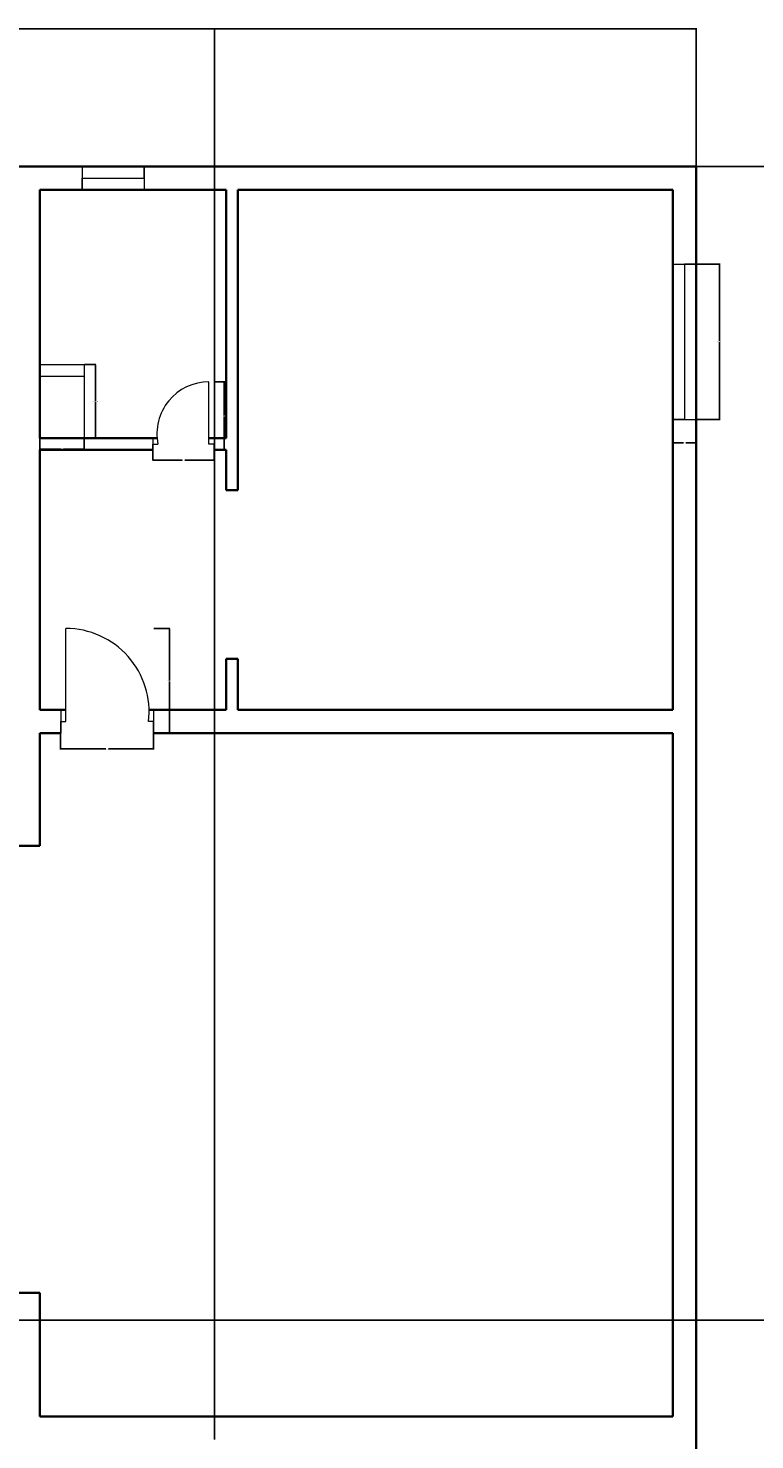
# Model space of a CAD drawing. Units: inches. Extents: x 2185 to 4426, y 1138 to 3073.
# Tile 12 of 14: x 3674 to 3955, y 1834 to 2380. Entities that reach past the tile are written whole.
import ezdxf

# ---------------------------------------------------------------- set-up
doc = ezdxf.new("R2010")
doc.units = ezdxf.units.IN
for name, color, linetype, lineweight in [('A-ANNO-DIMS', 2, 'Continuous', 18), ('A-ANNO-SYMB', 2, 'Continuous', 25), ('A-DOOR', 3, 'Continuous', 18), ('A-FLOR-CASE', 32, 'Continuous', 18), ('A-FURN', 8, 'Continuous', 18), ('A-GLAZ', 4, 'Continuous', 18), ('A-WALL', 7, 'Continuous', 35)]:
    doc.layers.add(name, color=color, linetype=linetype, lineweight=lineweight)
doc.styles.get("Standard").update_dxf_attribs({"font": 'arial.ttf'})
doc.dimstyles.get("Standard").update_dxf_attribs({"dimtxt": 0.18, "dimasz": 0.18, "dimexe": 0.18, "dimexo": 0.0625, "dimgap": 0.09, "dimtad": 0, "dimtih": 1, "dimtoh": 1, "dimdec": 4, "dimzin": 0, "dimdsep": 46, "dimtxsty": 'Standard', "dimcen": 0.09, "dimadec": 0, "dimazin": 0, "dimtfac": 1, "dimtdec": 4, "dimtofl": 0, "dimtmove": 0, "dimatfit": 3, "dimfxl": 1, "dimtolj": 1, "dimtzin": 0, "dimarcsym": 0})

# ---------------------------------------------------------------- blocks, each defined once
blk = doc.blocks.new('DOOR-SGL-24-ENSUITE')
for p, q in [((21.69, 2.25), (21.69, 26.25)), ((0, 4.5), (0, 0)), ((0, 0), (0, 2.25)), ((0, 2.25), (2, 2.25)), ((23.69, 2.25), (21.69, 2.25)), ((23.69, 4.5), (23.69, 0)), ((23.69, 0), (23.69, 2.25))]:
    blk.add_line(p, q)
blk.add_arc((21.69, 6.17), 20.08, 90, 191.26)
blk = doc.blocks.new('DOOR-SGL-36-BED-E')
for p, q in [((2, 4.5), (2, 40.5)), ((0, 9), (0, 0)), ((35.91, 9), (35.91, 0)), ((0, 0), (0, 4.5)), ((0, 4.5), (2, 4.5)), ((35.91, 4.5), (33.91, 4.5)), ((35.91, 0), (35.91, 4.5))]:
    blk.add_line(p, q)
blk.add_arc((2, 8.36), 32.14, 353.0978, 90)
blk = doc.blocks.new('WIN-PLAN-24IN-01')
for p, q in [((0, 9), (0, 0)), ((24, 4.5), (24, 9)), ((24, 9), (24, 0)), ((0, 0), (0, 4.5)), ((0, 4.5), (0, 4.5)), ((0, 4.5), (24, 4.5))]:
    blk.add_line(p, q)
blk = doc.blocks.new('WIN-PLAN-60IN-03')
for p, q in [((0, 60), (9, 60)), ((9, 60), (4.5, 60)), ((4.5, 60), (4.5, 0)), ((9, 60), (9, 60)), ((4.5, 0), (0, 0)), ((0, 0), (9, 0)), ((9, 0), (9, 0))]:
    blk.add_line(p, q)
blk = doc.blocks.new('BATH-CASEWORK')
for p, q in [((0, 28.5), (17.15, 28.5)), ((17.15, 28.5), (17.15, 0)), ((0, 24), (17.15, 24))]:
    blk.add_line(p, q)
blk = doc.blocks.new('*D62')
at = {"layer": 'A-ANNO-DIMS', "color": 0, "lineweight": -2, "transparency": 16777216}
for p, q in [((3746.18, 2243.13), (3750.24, 2243.13)), ((3750.06, 2242.95), (3750.06, 2230.19)), ((3750.06, 2217.06), (3750.06, 2229.82)), ((3746.18, 2216.88), (3750.24, 2216.88))]:
    blk.add_line(p, q, dxfattribs=at)
at = {"layer": 'A-ANNO-DIMS', "color": 0, "transparency": 16777216}
for points in [[(3750.03, 2242.95), (3750.09, 2242.95), (3750.06, 2243.13)], [(3750.03, 2217.06), (3750.09, 2217.06), (3750.06, 2216.88)]]:
    blk.add_solid(points, dxfattribs=at)
at = {"layer": 'Defpoints', "color": 0, "transparency": 16777216}
for p in [(3746.12, 2243.13), (3750.06, 2243.13), (3746.12, 2216.88)]:
    blk.add_point(p, dxfattribs=at)
at = {"layer": 'A-ANNO-DIMS', "color": 0, "transparency": 16777216, "insert": (3750.06, 2230), "char_height": 0.18, "attachment_point": 5}
blk.add_mtext('\\A1;DOOR 26 TYP.', dxfattribs=at)
blk = doc.blocks.new('*D63')
at = {"layer": 'A-ANNO-DIMS', "color": 0, "lineweight": -2, "transparency": 16777216}
for p, q in [((3722.43, 2216.81), (3722.43, 2212.76)), ((3746.12, 2216.81), (3746.12, 2212.76)), ((3722.61, 2212.94), (3733.74, 2212.94)), ((3745.94, 2212.94), (3734.8, 2212.94))]:
    blk.add_line(p, q, dxfattribs=at)
at = {"layer": 'A-ANNO-DIMS', "color": 0, "transparency": 16777216}
for points in [[(3722.61, 2212.97), (3722.61, 2212.91), (3722.43, 2212.94)], [(3745.94, 2212.97), (3745.94, 2212.91), (3746.12, 2212.94)]]:
    blk.add_solid(points, dxfattribs=at)
at = {"layer": 'Defpoints', "color": 0, "transparency": 16777216}
for p in [(3722.43, 2216.88), (3746.12, 2216.88), (3746.12, 2212.94)]:
    blk.add_point(p, dxfattribs=at)
at = {"layer": 'A-ANNO-DIMS', "color": 0, "transparency": 16777216, "insert": (3734.27, 2212.94), "char_height": 0.18, "attachment_point": 5}
blk.add_mtext('\\A1;24 TYP.', dxfattribs=at)
blk = doc.blocks.new('*D64')
at = {"layer": 'A-ANNO-DIMS', "color": 0, "lineweight": -2, "transparency": 16777216}
for p, q in [((3722.84, 2147.88), (3729.03, 2147.88)), ((3728.85, 2147.7), (3728.85, 2127.81)), ((3728.85, 2107.56), (3728.85, 2127.44)), ((3722.84, 2107.38), (3729.03, 2107.38))]:
    blk.add_line(p, q, dxfattribs=at)
at = {"layer": 'A-ANNO-DIMS', "color": 0, "transparency": 16777216}
for points in [[(3728.82, 2147.7), (3728.88, 2147.7), (3728.85, 2147.88)], [(3728.82, 2107.56), (3728.88, 2107.56), (3728.85, 2107.38)]]:
    blk.add_solid(points, dxfattribs=at)
at = {"layer": 'Defpoints', "color": 0, "transparency": 16777216}
for p in [(3722.78, 2147.88), (3728.85, 2147.88), (3722.78, 2107.38)]:
    blk.add_point(p, dxfattribs=at)
at = {"layer": 'A-ANNO-DIMS', "color": 0, "transparency": 16777216, "insert": (3728.85, 2127.63), "char_height": 0.18, "attachment_point": 5}
blk.add_mtext('\\A1;DOOR 41 TYP.', dxfattribs=at)
blk = doc.blocks.new('*D65')
at = {"layer": 'A-ANNO-DIMS', "color": 0, "lineweight": -2, "transparency": 16777216}
for p, q in [((3686.87, 2107.31), (3686.87, 2101.12)), ((3722.78, 2107.31), (3722.78, 2101.12)), ((3687.05, 2101.3), (3704.3, 2101.3)), ((3722.6, 2101.3), (3705.35, 2101.3))]:
    blk.add_line(p, q, dxfattribs=at)
at = {"layer": 'A-ANNO-DIMS', "color": 0, "transparency": 16777216}
for points in [[(3687.05, 2101.33), (3687.05, 2101.27), (3686.87, 2101.3)], [(3722.6, 2101.33), (3722.6, 2101.27), (3722.78, 2101.3)]]:
    blk.add_solid(points, dxfattribs=at)
at = {"layer": 'Defpoints', "color": 0, "transparency": 16777216}
for p in [(3686.87, 2107.38), (3722.78, 2107.38), (3722.78, 2101.3)]:
    blk.add_point(p, dxfattribs=at)
at = {"layer": 'A-ANNO-DIMS', "color": 0, "transparency": 16777216, "insert": (3704.83, 2101.3), "char_height": 0.18, "attachment_point": 5}
blk.add_mtext('\\A1;36 TYP.', dxfattribs=at)
blk = doc.blocks.new('*D108')
at = {"layer": 'A-ANNO-DIMS', "color": 0, "lineweight": -2, "transparency": 16777216}
for p, q in [((3932.41, 2288.64), (3941.53, 2288.64)), ((3941.35, 2288.46), (3941.35, 2258.83)), ((3941.35, 2228.82), (3941.35, 2258.46)), ((3932.41, 2228.64), (3941.53, 2228.64))]:
    blk.add_line(p, q, dxfattribs=at)
at = {"layer": 'A-ANNO-DIMS', "color": 0, "transparency": 16777216}
for points in [[(3941.32, 2288.46), (3941.38, 2288.46), (3941.35, 2288.64)], [(3941.32, 2228.82), (3941.38, 2228.82), (3941.35, 2228.64)]]:
    blk.add_solid(points, dxfattribs=at)
at = {"layer": 'Defpoints', "color": 0, "transparency": 16777216}
for p in [(3932.35, 2288.64), (3941.35, 2288.64), (3932.35, 2228.64)]:
    blk.add_point(p, dxfattribs=at)
at = {"layer": 'A-ANNO-DIMS', "color": 0, "transparency": 16777216, "insert": (3941.35, 2258.64), "char_height": 0.18, "attachment_point": 5}
blk.add_mtext('\\A1;WINDOW 60 TYP.', dxfattribs=at)
blk = doc.blocks.new('*D109')
at = {"layer": 'A-ANNO-DIMS', "color": 0, "lineweight": -2, "transparency": 16777216}
for p, q in [((3923.35, 2228.58), (3923.35, 2219.46)), ((3932.35, 2228.58), (3932.35, 2219.46)), ((3923.53, 2219.64), (3927.39, 2219.64)), ((3932.17, 2219.64), (3928.31, 2219.64))]:
    blk.add_line(p, q, dxfattribs=at)
at = {"layer": 'A-ANNO-DIMS', "color": 0, "transparency": 16777216}
for points in [[(3923.53, 2219.67), (3923.53, 2219.61), (3923.35, 2219.64)], [(3932.17, 2219.67), (3932.17, 2219.61), (3932.35, 2219.64)]]:
    blk.add_solid(points, dxfattribs=at)
at = {"layer": 'Defpoints', "color": 0, "transparency": 16777216}
for p in [(3923.35, 2228.64), (3932.35, 2228.64), (3932.35, 2219.64)]:
    blk.add_point(p, dxfattribs=at)
at = {"layer": 'A-ANNO-DIMS', "color": 0, "transparency": 16777216, "insert": (3927.85, 2219.64), "char_height": 0.18, "attachment_point": 5}
blk.add_mtext('\\A1;9 TYP.', dxfattribs=at)
blk = doc.blocks.new('*D124')
at = {"layer": 'A-ANNO-DIMS', "color": 0, "lineweight": -2, "transparency": 16777216}
for p, q in [((3696.06, 2249.88), (3700.45, 2249.88)), ((3700.27, 2249.7), (3700.27, 2235.81)), ((3700.27, 2221.56), (3700.27, 2235.44)), ((3696.06, 2221.38), (3700.45, 2221.38))]:
    blk.add_line(p, q, dxfattribs=at)
at = {"layer": 'A-ANNO-DIMS', "color": 0, "transparency": 16777216}
for points in [[(3700.24, 2249.7), (3700.3, 2249.7), (3700.27, 2249.88)], [(3700.24, 2221.56), (3700.3, 2221.56), (3700.27, 2221.38)]]:
    blk.add_solid(points, dxfattribs=at)
at = {"layer": 'Defpoints', "color": 0, "transparency": 16777216}
for p in [(3696, 2249.88), (3700.27, 2249.88), (3696, 2221.38)]:
    blk.add_point(p, dxfattribs=at)
at = {"layer": 'A-ANNO-DIMS', "color": 0, "transparency": 16777216, "insert": (3700.27, 2235.63), "char_height": 0.18, "attachment_point": 5}
blk.add_mtext('\\A1;BATH CABINET 29 TYP.', dxfattribs=at)
blk = doc.blocks.new('*D125')
at = {"layer": 'A-ANNO-DIMS', "color": 0, "lineweight": -2, "transparency": 16777216}
for p, q in [((3678.85, 2221.31), (3678.85, 2216.92)), ((3696, 2221.31), (3696, 2216.92)), ((3679.03, 2217.1), (3686.9, 2217.1)), ((3695.82, 2217.1), (3687.94, 2217.1))]:
    blk.add_line(p, q, dxfattribs=at)
at = {"layer": 'A-ANNO-DIMS', "color": 0, "transparency": 16777216}
for points in [[(3679.03, 2217.13), (3679.03, 2217.07), (3678.85, 2217.1)], [(3695.82, 2217.13), (3695.82, 2217.07), (3696, 2217.1)]]:
    blk.add_solid(points, dxfattribs=at)
at = {"layer": 'Defpoints', "color": 0, "transparency": 16777216}
for p in [(3678.85, 2221.38), (3696, 2221.38), (3696, 2217.1)]:
    blk.add_point(p, dxfattribs=at)
at = {"layer": 'A-ANNO-DIMS', "color": 0, "transparency": 16777216, "insert": (3687.42, 2217.1), "char_height": 0.18, "attachment_point": 5}
blk.add_mtext('\\A1;17 TYP.', dxfattribs=at)
blk = doc.blocks.new('*D145')
at = {"layer": 'A-ANNO-DIMS', "color": 0, "lineweight": -2, "transparency": 16777216}
for p, q in [((3210.85, 2326.44), (3210.85, 2379.81)), ((3211.03, 2379.63), (3571.21, 2379.63)), ((3932.17, 2379.63), (3571.99, 2379.63)), ((3932.35, 2326.44), (3932.35, 2379.81))]:
    blk.add_line(p, q, dxfattribs=at)
at = {"layer": 'A-ANNO-DIMS', "color": 0, "transparency": 16777216}
for points in [[(3211.03, 2379.66), (3211.03, 2379.6), (3210.85, 2379.63)], [(3932.17, 2379.66), (3932.17, 2379.6), (3932.35, 2379.63)]]:
    blk.add_solid(points, dxfattribs=at)
at = {"layer": 'Defpoints', "color": 0, "transparency": 16777216}
for p in [(3932.35, 2379.63), (3210.85, 2326.38), (3932.35, 2326.38)]:
    blk.add_point(p, dxfattribs=at)
at = {"layer": 'A-ANNO-DIMS', "color": 0, "transparency": 16777216, "insert": (3571.6, 2379.63), "char_height": 0.18, "attachment_point": 5}
blk.add_mtext('\\A1;721.5', dxfattribs=at)
blk = doc.blocks.new('*D146')
at = {"layer": 'A-ANNO-DIMS', "color": 0, "lineweight": -2, "transparency": 16777216}
for p, q in [((3932.41, 2326.38), (4058.64, 2326.38)), ((4058.46, 2326.2), (4058.46, 1827.06)), ((4058.46, 1327.56), (4058.46, 1826.7)), ((3932.41, 1327.38), (4058.64, 1327.38))]:
    blk.add_line(p, q, dxfattribs=at)
at = {"layer": 'A-ANNO-DIMS', "color": 0, "transparency": 16777216}
for points in [[(4058.43, 2326.2), (4058.49, 2326.2), (4058.46, 2326.38)], [(4058.43, 1327.56), (4058.49, 1327.56), (4058.46, 1327.38)]]:
    blk.add_solid(points, dxfattribs=at)
at = {"layer": 'Defpoints', "color": 0, "transparency": 16777216}
for p in [(3932.35, 2326.38), (4058.46, 2326.38), (3932.35, 1327.38)]:
    blk.add_point(p, dxfattribs=at)
at = {"layer": 'A-ANNO-DIMS', "color": 0, "transparency": 16777216, "insert": (4058.46, 1826.88), "char_height": 0.18, "attachment_point": 5}
blk.add_mtext('\\A1;999', dxfattribs=at)
blk = doc.blocks.new('*D157')
at = {"layer": 'A-ANNO-DIMS', "color": 0, "lineweight": -2, "transparency": 16777216}
for p, q in [((3665.35, 1753.44), (3665.35, 2379.81)), ((3665.53, 2379.63), (3705.65, 2379.63)), ((3746.17, 2379.63), (3706.05, 2379.63)), ((3746.35, 1834.44), (3746.35, 2379.81))]:
    blk.add_line(p, q, dxfattribs=at)
at = {"layer": 'A-ANNO-DIMS', "color": 0, "transparency": 16777216}
for points in [[(3665.53, 2379.66), (3665.53, 2379.6), (3665.35, 2379.63)], [(3746.17, 2379.66), (3746.17, 2379.6), (3746.35, 2379.63)]]:
    blk.add_solid(points, dxfattribs=at)
at = {"layer": 'Defpoints', "color": 0, "transparency": 16777216}
for p in [(3746.35, 2379.63), (3746.35, 1834.38), (3665.35, 1753.38)]:
    blk.add_point(p, dxfattribs=at)
at = {"layer": 'A-ANNO-DIMS', "color": 0, "transparency": 16777216, "insert": (3705.85, 2379.63), "char_height": 0.18, "attachment_point": 5}
blk.add_mtext('\\A1;81', dxfattribs=at)

msp = doc.modelspace()

# ---------------------------------------------------------------- linework, layer by layer
at = {"layer": 'A-ANNO-SYMB'}
msp.add_line((3155.074, 1880.563), (4005.21, 1880.563), dxfattribs=at)
at = {"layer": 'A-FURN', "ltscale": 0.03}
for p, q in [((3923.349, 2037.715), (3923.349, 1937.955)), ((3923.349, 2037.715), (3923.349, 1937.955)), ((3923.349, 2034.921), (3923.349, 1940.75)), ((3923.349, 2034.921), (3923.349, 1940.75))]:
    msp.add_line(p, q, dxfattribs=at)
at = {"layer": 'A-WALL'}
for p, q in [((3210.849, 2326.377), (3932.349, 2326.377)), ((3210.849, 2326.377), (3932.349, 2326.377)), ((3932.349, 2326.377), (3932.349, 1327.377)), ((3932.349, 2326.377), (3932.349, 1327.377)), ((3678.849, 2317.377), (3678.849, 2221.377)), ((3678.849, 2317.377), (3750.849, 2317.377)), ((3678.849, 2317.377), (3678.849, 2221.377)), ((3678.849, 2317.377), (3750.849, 2317.377)), ((3750.849, 2317.377), (3750.849, 2221.377)), ((3750.849, 2317.377), (3750.849, 2221.377)), ((3755.349, 2317.377), (3755.349, 2201.367)), ((3755.349, 2317.377), (3923.349, 2317.377)), ((3755.349, 2317.377), (3755.349, 2201.367)), ((3755.349, 2317.377), (3923.349, 2317.377)), ((3923.349, 2317.377), (3923.349, 2116.377)), ((3923.349, 2317.377), (3923.349, 2116.377)), ((3678.849, 2221.377), (3724.109, 2221.377)), ((3678.849, 2221.377), (3724.109, 2221.377)), ((3744.119, 2221.377), (3750.849, 2221.377)), ((3744.119, 2221.377), (3750.849, 2221.377)), ((3678.849, 2216.877), (3678.849, 2116.377)), ((3678.849, 2216.877), (3722.426, 2216.877)), ((3678.849, 2216.877), (3678.849, 2116.377)), ((3678.849, 2216.877), (3722.426, 2216.877)), ((3746.119, 2216.877), (3750.849, 2216.877)), ((3746.119, 2216.877), (3750.849, 2216.877)), ((3750.849, 2216.877), (3750.849, 2201.367)), ((3750.849, 2216.877), (3750.849, 2201.367)), ((3750.849, 2201.367), (3755.349, 2201.367)), ((3750.849, 2201.367), (3755.349, 2201.367)), ((3750.849, 2136.181), (3750.849, 2116.377)), ((3750.849, 2136.181), (3755.349, 2136.181)), ((3750.849, 2136.181), (3750.849, 2116.377)), ((3750.849, 2136.181), (3755.349, 2136.181)), ((3755.349, 2136.181), (3755.349, 2116.377)), ((3755.349, 2136.181), (3755.349, 2116.377)), ((3678.849, 2116.377), (3688.874, 2116.377)), ((3678.849, 2116.377), (3688.874, 2116.377)), ((3721.006, 2116.377), (3750.849, 2116.377)), ((3721.006, 2116.377), (3750.849, 2116.377)), ((3755.349, 2116.377), (3923.349, 2116.377)), ((3755.349, 2116.377), (3923.349, 2116.377)), ((3678.849, 2107.377), (3678.849, 2063.852)), ((3678.849, 2107.377), (3686.874, 2107.377)), ((3678.849, 2107.377), (3678.849, 2063.852)), ((3678.849, 2107.377), (3686.874, 2107.377)), ((3722.779, 2107.377), (3923.349, 2107.377)), ((3722.779, 2107.377), (3923.349, 2107.377)), ((3923.349, 2107.377), (3923.349, 1843.377)), ((3923.349, 2107.377), (3923.349, 1843.377)), ((3669.849, 2063.852), (3678.849, 2063.852)), ((3669.849, 2063.852), (3678.849, 2063.852)), ((3669.849, 1891.155), (3678.849, 1891.155)), ((3669.849, 1891.155), (3678.849, 1891.155)), ((3678.849, 1891.155), (3678.849, 1843.377)), ((3678.849, 1891.155), (3678.849, 1843.377)), ((3678.849, 1843.377), (3923.349, 1843.377)), ((3678.849, 1843.377), (3923.349, 1843.377)), ((3678.849, 1843.377), (3923.349, 1843.377)), ((3678.849, 1843.377), (3923.349, 1843.377))]:
    msp.add_line(p, q, dxfattribs=at)

# ---------------------------------------------------------------- block references
at = {"layer": 'A-DOOR'}
for name, p in [('DOOR-SGL-24-ENSUITE', (3722.426, 2216.877)), ('DOOR-SGL-24-ENSUITE', (3722.426, 2216.877)), ('DOOR-SGL-36-BED-E', (3686.874, 2107.377)), ('DOOR-SGL-36-BED-E', (3686.874, 2107.377))]:
    msp.add_blockref(name, p, dxfattribs=at)
at = {"layer": 'A-FLOR-CASE'}
msp.add_blockref('BATH-CASEWORK', (3678.849, 2221.377), dxfattribs=at)
msp.add_blockref('BATH-CASEWORK', (3678.849, 2221.377), dxfattribs=at)
at = {"layer": 'A-GLAZ'}
for name, p in [('WIN-PLAN-24IN-01', (3695.178, 2317.377)), ('WIN-PLAN-24IN-01', (3695.178, 2317.377)), ('WIN-PLAN-60IN-03', (3923.349, 2228.643)), ('WIN-PLAN-60IN-03', (3923.349, 2228.643))]:
    msp.add_blockref(name, p, dxfattribs=at)

# ---------------------------------------------------------------- dimensions: what is measured, and where the dimension line sits
at = {"layer": 'A-ANNO-DIMS'}
for base, p1, p2, override, picture, middle in [((3932.349, 2379.627), (3210.849, 2326.377), (3932.349, 2326.377), {"dimdec": 1, "dimlfac": 1, "dimrnd": 0, "dimzin": 0, "dimdsep": 46, "dimlunit": 2}, '*D145', (3571.599, 2379.627)), ((3746.349, 2379.627), (3665.349, 1753.377), (3746.349, 1834.377), {"dimdec": 0, "dimlfac": 1, "dimrnd": 0, "dimzin": 0, "dimdsep": 46, "dimlunit": 2}, '*D157', (3705.849, 2379.627))]:
    dim = msp.add_linear_dim(base=base, p1=p1, p2=p2, dimstyle='Standard', override=override, dxfattribs=at)
    dim.commit()
    dim.dimension.update_dxf_attribs({"geometry": picture, "text_midpoint": middle})
dim = msp.add_linear_dim(base=(4058.46, 2326.377), p1=(3932.349, 1327.377), p2=(3932.349, 2326.377), angle=90, dimstyle='Standard', override={"dimdec": 0, "dimlfac": 1, "dimrnd": 0, "dimzin": 0, "dimdsep": 46, "dimlunit": 2}, dxfattribs=at)
dim.commit()
dim.dimension.update_dxf_attribs({"geometry": '*D146', "text_midpoint": (4058.46, 1826.877)})
for base, p1, p2, text, picture, middle in [((3941.349, 2288.643), (3932.349, 2228.643), (3932.349, 2288.643), 'WINDOW <> TYP.', '*D108', (3941.349, 2258.643)), ((3700.272876897, 2249.876947079), (3695.997876897, 2221.376947079), (3695.997876897, 2249.876947079), 'BATH CABINET <> TYP.', '*D124', (3700.272876897, 2235.626947079)), ((3750.056, 2243.127), (3746.119, 2216.877), (3746.119, 2243.127), 'DOOR <> TYP.', '*D62', (3750.056, 2230.002)), ((3728.854146907, 2147.876947079), (3722.779146907, 2107.376947079), (3722.779146907, 2147.876947079), 'DOOR <> TYP.', '*D64', (3728.854146907, 2127.626947079))]:
    dim = msp.add_linear_dim(base=base, p1=p1, p2=p2, angle=90, text=text, dimstyle='Standard', override={"dimdec": 0, "dimlfac": 1, "dimrnd": 0, "dimzin": 0, "dimdsep": 46, "dimlunit": 2}, dxfattribs=at)
    dim.commit()
    dim.dimension.update_dxf_attribs({"geometry": picture, "text_midpoint": middle})
for base, p1, p2, picture, middle in [((3932.349, 2219.643), (3923.349, 2228.643), (3932.349, 2228.643), '*D109', (3927.849, 2219.643)), ((3695.998, 2217.102), (3678.849, 2221.377), (3695.998, 2221.377), '*D125', (3687.424, 2217.102)), ((3746.119, 2212.939), (3722.426, 2216.877), (3746.119, 2216.877), '*D63', (3734.272, 2212.939)), ((3722.779, 2101.302), (3686.874, 2107.377), (3722.779, 2107.377), '*D65', (3704.827, 2101.302))]:
    dim = msp.add_linear_dim(base=base, p1=p1, p2=p2, text='<> TYP.', dimstyle='Standard', override={"dimdec": 0, "dimlfac": 1, "dimrnd": 0, "dimzin": 0, "dimdsep": 46, "dimlunit": 2}, dxfattribs=at)
    dim.commit()
    dim.dimension.update_dxf_attribs({"geometry": picture, "text_midpoint": middle})

doc.saveas('drawing.dxf')
